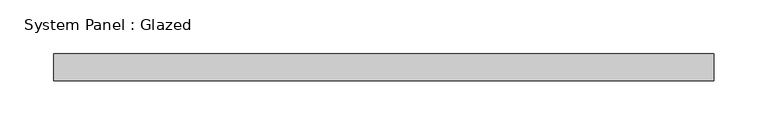
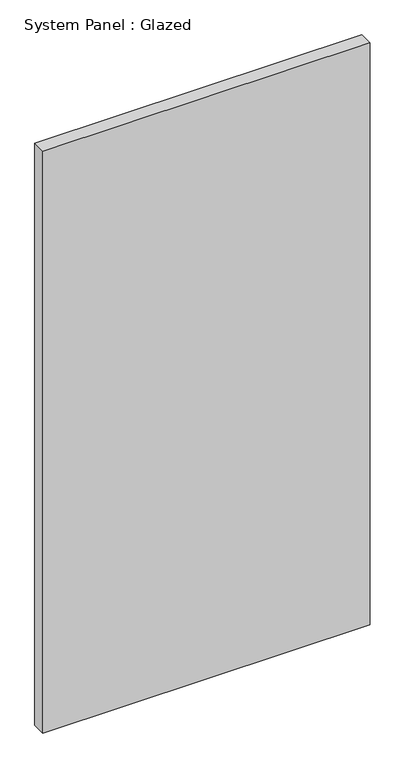
"""IFC4 building model written with IfcOpenShell, lengths in millimetres: plate geometry, System Panel : Glazed."""

from ifc_helpers import new_model, si_unit, origin, origin_with_axes, place, context, project, spatial, polyline, outline, extrude, source, transform, mapped, element, save


def system_panel_glazed_3baf32ff(model_context):
    return source(origin(), model_context, "Body", "SweptSolid", [
        extrude(outline(polyline([(307.4713738, 19.05), (-307.4713738, 19.05), (-307.4713738, 44.45), (307.4713738, 44.45), (307.4713738, 19.05)])), origin_with_axes(), (0.0, 0.0, 1.0), 1155.7),
    ])


if __name__ == "__main__":
    model = new_model("IFC4")
    model_context = context("Model", 3, world=origin())
    ifc_project = project(units=[si_unit("LENGTHUNIT", "METRE", prefix="MILLI")], contexts=[model_context])
    site = spatial("IfcSite", under=ifc_project)
    building = spatial("IfcBuilding", under=site)
    placement = place(None, origin())
    system_panel_glazed_shape = system_panel_glazed_3baf32ff(model_context)
    element("IfcPlate", 1, ObjectType="System Panel : Glazed", at=placement, inside=building, context=model_context, shape_type="MappedRepresentation", body=[
        mapped(system_panel_glazed_shape, transform((0.0, 0.0, 0.0), x_axis=(1.0, 0.0, 0.0), y_axis=(0.0, 1.0, 0.0), z_axis=(0.0, 0.0, 1.0))),
    ])
    save(model, "model.ifc")

# Revit data of these elements
# Type "System Panel : Glazed"
#   Construction Type Id = "GSP4R"
#   Analytic Construction = "1/8 in Pilkington single glazing"
#   Visual Light Transmittance = 0.9
#   Solar Heat Gain Coefficient = 0.86
#   Heat Transfer Coefficient (U) = 1.18115 BTU/(h·ft²·°F)
# Element 1 (IfcPlate, "System Panel : Glazed")
#   Materials on its faces: "Glass"
# Materials
#   "Glass": class "Glass", colour RGB 0 128 192, transparency 0.75, Description = "Soda Lime Glass", Cost = 0
